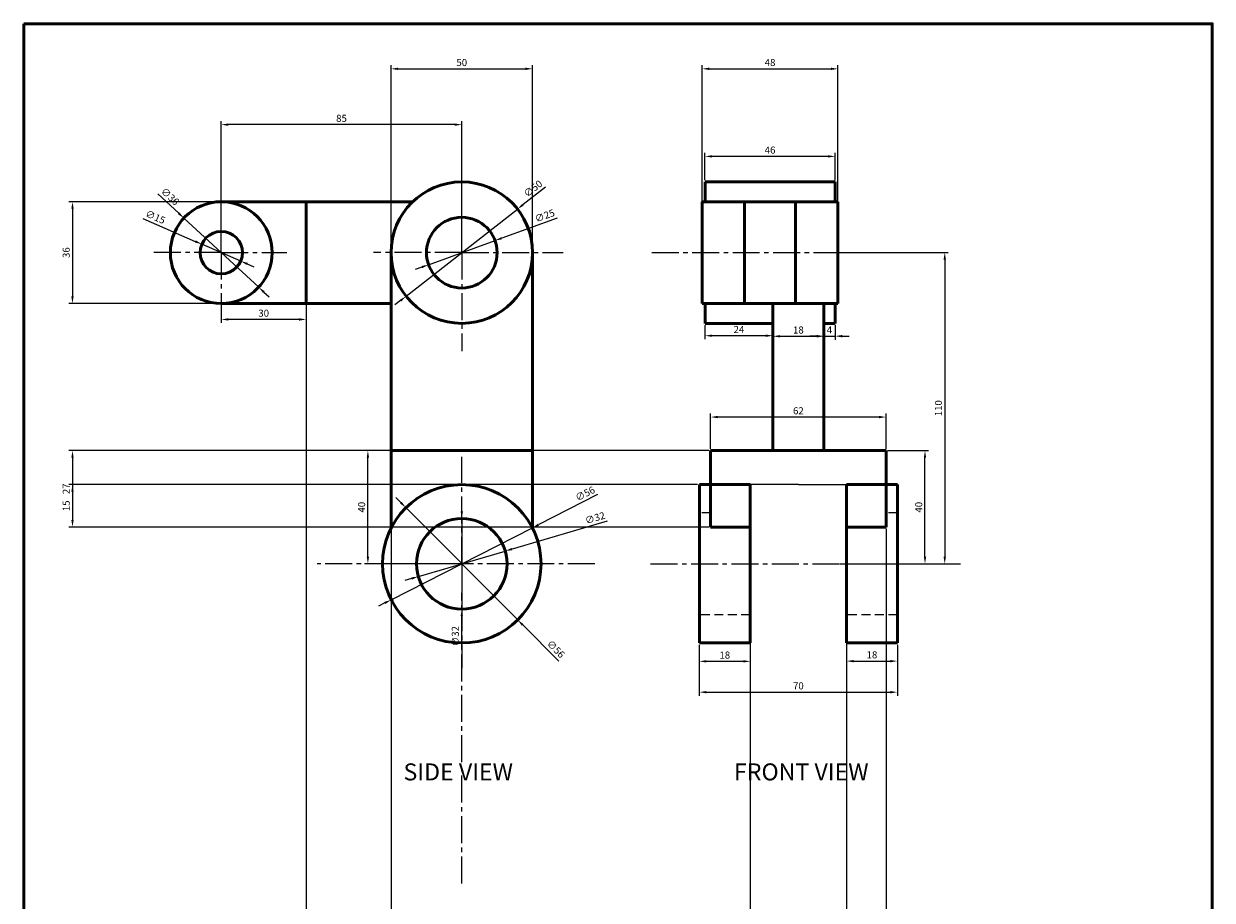
# Model space of a CAD drawing. Units: millimetres. Extents: x 1466 to 1886, y 5011 to 5605.
# Tile 4 of 4: x 1466 to 1886, y 5295 to 5605. Entities that reach past the tile are written whole.
import ezdxf

# ---------------------------------------------------------------- set-up
doc = ezdxf.new("R2010")
doc.units = ezdxf.units.MM
doc.linetypes.add('CENTER2', pattern=[28.575, 19.05, -3.175, 3.175, -3.175])
doc.linetypes.add('HIDDEN2', pattern=[4.7625, 3.175, -1.5875])
for name, color, linetype, lineweight in [('M-CNTR', 1, 'CENTER2', 18), ('M-DIMS', 2, 'Continuous', 25), ('M-HIDN', 4, 'HIDDEN2', 25), ('M-OUTL', 7, 'Continuous', 50), ('M-TEXT', 7, 'Continuous', 25), ('M-TTLB', 7, 'Continuous', 50)]:
    doc.layers.add(name, color=color, linetype=linetype, lineweight=lineweight)
doc.styles.get("Standard").update_dxf_attribs({"font": 'arial.ttf'})
doc.dimstyles.new('ISO-25', dxfattribs={"dimtxt": 2.5, "dimasz": 2.5, "dimexe": 1.25, "dimexo": 0.625, "dimtad": 1, "dimtxsty": 'Standard', "dimcen": 2.5, "dimadec": 0, "dimazin": 0, "dimtfac": 1, "dimtmove": 0, "dimatfit": 3, "dimfxl": 1, "dimarcsym": 0})

# ---------------------------------------------------------------- blocks, each defined once
blk = doc.blocks.new('*D26')
at = {"layer": 'Defpoints', "color": 0, "transparency": 16777216}
for p in [(1707.01, 5557.74), (1707.01, 5548.72), (1753.01, 5548.72)]:
    blk.add_point(p, dxfattribs=at)
at = {"layer": 'M-DIMS', "color": 0, "lineweight": -2, "transparency": 16777216}
for p, q in [((1707.01, 5549.34), (1707.01, 5558.99)), ((1750.51, 5557.74), (1709.51, 5557.74)), ((1753.01, 5549.34), (1753.01, 5558.99))]:
    blk.add_line(p, q, dxfattribs=at)
at = {"layer": 'M-DIMS', "color": 0, "transparency": 16777216}
for points in [[(1709.51, 5558.16), (1709.51, 5557.33), (1707.01, 5557.74)], [(1750.51, 5558.16), (1750.51, 5557.33), (1753.01, 5557.74)]]:
    blk.add_solid(points, dxfattribs=at)
at = {"layer": 'M-DIMS', "color": 0, "transparency": 16777216, "insert": (1730.01, 5559.65), "char_height": 2.5, "attachment_point": 5}
blk.add_mtext('46', dxfattribs=at)
blk = doc.blocks.new('*D27')
at = {"layer": 'Defpoints', "color": 0, "transparency": 16777216}
for p in [(1754.01, 5523.72), (1754.01, 5413.72), (1791.74, 5413.72)]:
    blk.add_point(p, dxfattribs=at)
at = {"layer": 'M-DIMS', "color": 0, "lineweight": -2, "transparency": 16777216}
for p, q in [((1754.64, 5523.72), (1792.99, 5523.72)), ((1791.74, 5521.22), (1791.74, 5416.22)), ((1754.64, 5413.72), (1792.99, 5413.72))]:
    blk.add_line(p, q, dxfattribs=at)
at = {"layer": 'M-DIMS', "color": 0, "transparency": 16777216}
for points in [[(1791.32, 5521.22), (1792.16, 5521.22), (1791.74, 5523.72)], [(1791.32, 5416.22), (1792.16, 5416.22), (1791.74, 5413.72)]]:
    blk.add_solid(points, dxfattribs=at)
at = {"layer": 'M-DIMS', "color": 0, "transparency": 16777216, "insert": (1789.84, 5468.72), "char_height": 2.5, "attachment_point": 5, "rotation": 90}
blk.add_mtext('110', dxfattribs=at)
blk = doc.blocks.new('*D28')
at = {"layer": 'Defpoints', "color": 0, "transparency": 16777216}
for p in [(1709.01, 5465.59), (1709.01, 5453.72), (1771.01, 5453.72)]:
    blk.add_point(p, dxfattribs=at)
at = {"layer": 'M-DIMS', "color": 0, "lineweight": -2, "transparency": 16777216}
for p, q in [((1709.01, 5454.34), (1709.01, 5466.84)), ((1768.51, 5465.59), (1711.51, 5465.59)), ((1771.01, 5454.34), (1771.01, 5466.84))]:
    blk.add_line(p, q, dxfattribs=at)
at = {"layer": 'M-DIMS', "color": 0, "transparency": 16777216}
for points in [[(1711.51, 5466), (1711.51, 5465.17), (1709.01, 5465.59)], [(1768.51, 5466), (1768.51, 5465.17), (1771.01, 5465.59)]]:
    blk.add_solid(points, dxfattribs=at)
at = {"layer": 'M-DIMS', "color": 0, "transparency": 16777216, "insert": (1740.01, 5467.49), "char_height": 2.5, "attachment_point": 5}
blk.add_mtext('62', dxfattribs=at)
blk = doc.blocks.new('*D29')
at = {"layer": 'Defpoints', "color": 0, "transparency": 16777216}
for p in [(1705.01, 5385.72), (1723.01, 5385.72), (1705.01, 5379.23)]:
    blk.add_point(p, dxfattribs=at)
at = {"layer": 'M-DIMS', "color": 0, "lineweight": -2, "transparency": 16777216}
for p, q in [((1705.01, 5385.09), (1705.01, 5377.98)), ((1723.01, 5385.09), (1723.01, 5377.98)), ((1720.51, 5379.23), (1707.51, 5379.23))]:
    blk.add_line(p, q, dxfattribs=at)
at = {"layer": 'M-DIMS', "color": 0, "transparency": 16777216}
for points in [[(1707.51, 5379.65), (1707.51, 5378.81), (1705.01, 5379.23)], [(1720.51, 5379.65), (1720.51, 5378.81), (1723.01, 5379.23)]]:
    blk.add_solid(points, dxfattribs=at)
at = {"layer": 'M-DIMS', "color": 0, "transparency": 16777216, "insert": (1714.01, 5381.13), "char_height": 2.5, "attachment_point": 5}
blk.add_mtext('18', dxfattribs=at)
blk = doc.blocks.new('*D30')
at = {"layer": 'Defpoints', "color": 0, "transparency": 16777216}
for p in [(1757.01, 5385.72), (1775.01, 5385.72), (1775.01, 5379.31)]:
    blk.add_point(p, dxfattribs=at)
at = {"layer": 'M-DIMS', "color": 0, "lineweight": -2, "transparency": 16777216}
for p, q in [((1757.01, 5385.09), (1757.01, 5378.06)), ((1775.01, 5385.09), (1775.01, 5378.06)), ((1759.51, 5379.31), (1772.51, 5379.31))]:
    blk.add_line(p, q, dxfattribs=at)
at = {"layer": 'M-DIMS', "color": 0, "transparency": 16777216}
for points in [[(1759.51, 5379.72), (1759.51, 5378.89), (1757.01, 5379.31)], [(1772.51, 5379.72), (1772.51, 5378.89), (1775.01, 5379.31)]]:
    blk.add_solid(points, dxfattribs=at)
at = {"layer": 'M-DIMS', "color": 0, "transparency": 16777216, "insert": (1766.01, 5381.21), "char_height": 2.5, "attachment_point": 5}
blk.add_mtext('18', dxfattribs=at)
blk = doc.blocks.new('*D31')
at = {"layer": 'Defpoints', "color": 0, "transparency": 16777216}
for p in [(1705.01, 5385.72), (1775.01, 5385.72), (1775.01, 5368.33)]:
    blk.add_point(p, dxfattribs=at)
at = {"layer": 'M-DIMS', "color": 0, "lineweight": -2, "transparency": 16777216}
for p, q in [((1705.01, 5385.09), (1705.01, 5367.08)), ((1775.01, 5385.09), (1775.01, 5367.08)), ((1707.51, 5368.33), (1772.51, 5368.33))]:
    blk.add_line(p, q, dxfattribs=at)
at = {"layer": 'M-DIMS', "color": 0, "transparency": 16777216}
for points in [[(1707.51, 5368.74), (1707.51, 5367.91), (1705.01, 5368.33)], [(1772.51, 5368.74), (1772.51, 5367.91), (1775.01, 5368.33)]]:
    blk.add_solid(points, dxfattribs=at)
at = {"layer": 'M-DIMS', "color": 0, "transparency": 16777216, "insert": (1740.01, 5370.23), "char_height": 2.5, "attachment_point": 5}
blk.add_mtext('70', dxfattribs=at)
blk = doc.blocks.new('*D32')
at = {"layer": 'Defpoints', "color": 0, "transparency": 16777216}
for p in [(1771.01, 5453.72), (1784.76, 5453.72), (1775.01, 5413.72)]:
    blk.add_point(p, dxfattribs=at)
at = {"layer": 'M-DIMS', "color": 0, "lineweight": -2, "transparency": 16777216}
for p, q in [((1771.64, 5453.72), (1786.01, 5453.72)), ((1784.76, 5416.22), (1784.76, 5451.22)), ((1775.64, 5413.72), (1786.01, 5413.72))]:
    blk.add_line(p, q, dxfattribs=at)
at = {"layer": 'M-DIMS', "color": 0, "transparency": 16777216}
for points in [[(1784.35, 5451.22), (1785.18, 5451.22), (1784.76, 5453.72)], [(1784.35, 5416.22), (1785.18, 5416.22), (1784.76, 5413.72)]]:
    blk.add_solid(points, dxfattribs=at)
at = {"layer": 'M-DIMS', "color": 0, "transparency": 16777216, "insert": (1782.86, 5433.72), "char_height": 2.5, "attachment_point": 5, "rotation": 90}
blk.add_mtext('40', dxfattribs=at)
blk = doc.blocks.new('*D33')
at = {"layer": 'Defpoints', "color": 0, "transparency": 16777216}
for p in [(1707.01, 5498.72), (1731.01, 5498.72), (1707.01, 5494.35)]:
    blk.add_point(p, dxfattribs=at)
at = {"layer": 'M-DIMS', "color": 0, "lineweight": -2, "transparency": 16777216}
for p, q in [((1707.01, 5498.09), (1707.01, 5493.1)), ((1731.01, 5498.09), (1731.01, 5493.1)), ((1728.51, 5494.35), (1709.51, 5494.35))]:
    blk.add_line(p, q, dxfattribs=at)
at = {"layer": 'M-DIMS', "color": 0, "transparency": 16777216}
for points in [[(1709.51, 5494.77), (1709.51, 5493.94), (1707.01, 5494.35)], [(1728.51, 5494.77), (1728.51, 5493.94), (1731.01, 5494.35)]]:
    blk.add_solid(points, dxfattribs=at)
at = {"layer": 'M-DIMS', "color": 0, "transparency": 16777216, "insert": (1719.01, 5496.23), "char_height": 2.5, "attachment_point": 5}
blk.add_mtext('24', dxfattribs=at)
blk = doc.blocks.new('*D34')
at = {"layer": 'Defpoints', "color": 0, "transparency": 16777216}
for p in [(1731.01, 5498.72), (1749.01, 5498.72), (1749.01, 5494.15)]:
    blk.add_point(p, dxfattribs=at)
at = {"layer": 'M-DIMS', "color": 0, "lineweight": -2, "transparency": 16777216}
for p, q in [((1731.01, 5498.09), (1731.01, 5492.9)), ((1749.01, 5498.09), (1749.01, 5492.9)), ((1733.51, 5494.15), (1746.51, 5494.15))]:
    blk.add_line(p, q, dxfattribs=at)
at = {"layer": 'M-DIMS', "color": 0, "transparency": 16777216}
for points in [[(1733.51, 5494.56), (1733.51, 5493.73), (1731.01, 5494.15)], [(1746.51, 5494.56), (1746.51, 5493.73), (1749.01, 5494.15)]]:
    blk.add_solid(points, dxfattribs=at)
at = {"layer": 'M-DIMS', "color": 0, "transparency": 16777216, "insert": (1740.01, 5496.05), "char_height": 2.5, "attachment_point": 5}
blk.add_mtext('18', dxfattribs=at)
blk = doc.blocks.new('*D35')
at = {"layer": 'Defpoints', "color": 0, "transparency": 16777216}
for p in [(1749.01, 5498.72), (1753.01, 5498.72), (1753.01, 5494.19)]:
    blk.add_point(p, dxfattribs=at)
at = {"layer": 'M-DIMS', "color": 0, "lineweight": -2, "transparency": 16777216}
for p, q in [((1749.01, 5498.09), (1749.01, 5492.94)), ((1753.01, 5498.09), (1753.01, 5492.94)), ((1746.51, 5494.19), (1744.01, 5494.19)), ((1749.01, 5494.19), (1753.01, 5494.19)), ((1755.51, 5494.19), (1758.01, 5494.19))]:
    blk.add_line(p, q, dxfattribs=at)
at = {"layer": 'M-DIMS', "color": 0, "transparency": 16777216}
for points in [[(1746.51, 5494.61), (1746.51, 5493.77), (1749.01, 5494.19)], [(1755.51, 5494.61), (1755.51, 5493.77), (1753.01, 5494.19)]]:
    blk.add_solid(points, dxfattribs=at)
at = {"layer": 'M-DIMS', "color": 0, "transparency": 16777216, "insert": (1751.01, 5496.06), "char_height": 2.5, "attachment_point": 5}
blk.add_mtext('4', dxfattribs=at)
blk = doc.blocks.new('*D36')
at = {"layer": 'Defpoints', "color": 0, "transparency": 16777216}
for p in [(1522.85, 5535.94), (1549.28, 5511.49)]:
    blk.add_point(p, dxfattribs=at)
at = {"layer": 'M-DIMS', "color": 0, "lineweight": -2, "transparency": 16777216}
for p, q in [((1513.64, 5544.46), (1521.02, 5537.64)), ((1549.28, 5511.49), (1522.85, 5535.94)), ((1551.11, 5509.79), (1552.95, 5508.1))]:
    blk.add_line(p, q, dxfattribs=at)
at = {"layer": 'M-DIMS', "color": 0, "transparency": 16777216}
for points in [[(1521.3, 5537.94), (1520.73, 5537.33), (1522.85, 5535.94)], [(1551.4, 5510.1), (1550.83, 5509.49), (1549.28, 5511.49)]]:
    blk.add_solid(points, dxfattribs=at)
at = {"layer": 'M-DIMS', "color": 0, "transparency": 16777216, "insert": (1517.75, 5543.35), "char_height": 2.5, "attachment_point": 5, "rotation": 317.2254}
blk.add_mtext('∅36', dxfattribs=at)
blk = doc.blocks.new('*D37')
at = {"layer": 'Defpoints', "color": 0, "transparency": 16777216}
for p in [(1529.19, 5526.7), (1542.94, 5520.73)]:
    blk.add_point(p, dxfattribs=at)
at = {"layer": 'M-DIMS', "color": 0, "lineweight": -2, "transparency": 16777216}
for p, q in [((1508.4, 5535.73), (1526.89, 5527.7)), ((1542.94, 5520.73), (1529.19, 5526.7)), ((1545.24, 5519.73), (1547.53, 5518.74))]:
    blk.add_line(p, q, dxfattribs=at)
at = {"layer": 'M-DIMS', "color": 0, "transparency": 16777216}
for points in [[(1527.06, 5528.08), (1526.73, 5527.32), (1529.19, 5526.7)], [(1545.4, 5520.12), (1545.07, 5519.35), (1542.94, 5520.73)]]:
    blk.add_solid(points, dxfattribs=at)
at = {"layer": 'M-DIMS', "color": 0, "transparency": 16777216, "insert": (1512.66, 5536.03), "char_height": 2.5, "attachment_point": 5, "rotation": 336.5262}
blk.add_mtext('∅15', dxfattribs=at)
blk = doc.blocks.new('*D38')
at = {"layer": 'Defpoints', "color": 0, "transparency": 16777216}
for p in [(1640.74, 5539.13), (1601.39, 5508.3)]:
    blk.add_point(p, dxfattribs=at)
at = {"layer": 'M-DIMS', "color": 0, "lineweight": -2, "transparency": 16777216}
for p, q in [((1650.62, 5546.87), (1642.71, 5540.68)), ((1601.39, 5508.3), (1640.74, 5539.13)), ((1599.42, 5506.76), (1597.45, 5505.21))]:
    blk.add_line(p, q, dxfattribs=at)
at = {"layer": 'M-DIMS', "color": 0, "transparency": 16777216}
for points in [[(1642.46, 5541), (1642.97, 5540.35), (1640.74, 5539.13)], [(1599.16, 5507.08), (1599.67, 5506.43), (1601.39, 5508.3)]]:
    blk.add_solid(points, dxfattribs=at)
at = {"layer": 'M-DIMS', "color": 0, "transparency": 16777216, "insert": (1646.43, 5546.1), "char_height": 2.5, "attachment_point": 5, "rotation": 38.0777}
blk.add_mtext('∅50', dxfattribs=at)
blk = doc.blocks.new('*D39')
at = {"layer": 'Defpoints', "color": 0, "transparency": 16777216}
for p in [(1632.82, 5527.98), (1609.31, 5519.46)]:
    blk.add_point(p, dxfattribs=at)
at = {"layer": 'M-DIMS', "color": 0, "lineweight": -2, "transparency": 16777216}
for p, q in [((1654.71, 5535.91), (1635.17, 5528.83)), ((1609.31, 5519.46), (1632.82, 5527.98)), ((1606.96, 5518.61), (1604.61, 5517.75))]:
    blk.add_line(p, q, dxfattribs=at)
at = {"layer": 'M-DIMS', "color": 0, "transparency": 16777216}
for points in [[(1635.03, 5529.22), (1635.31, 5528.44), (1632.82, 5527.98)], [(1606.82, 5519), (1607.1, 5518.21), (1609.31, 5519.46)]]:
    blk.add_solid(points, dxfattribs=at)
at = {"layer": 'M-DIMS', "color": 0, "transparency": 16777216, "insert": (1650.48, 5536.47), "char_height": 2.5, "attachment_point": 5, "rotation": 19.9205}
blk.add_mtext('∅25', dxfattribs=at)
blk = doc.blocks.new('*D40')
at = {"layer": 'Defpoints', "color": 0, "transparency": 16777216}
for p in [(1646.01, 5426.43), (1596.12, 5401)]:
    blk.add_point(p, dxfattribs=at)
at = {"layer": 'M-DIMS', "color": 0, "lineweight": -2, "transparency": 16777216}
for p, q in [((1669.04, 5438.18), (1648.24, 5427.57)), ((1596.12, 5401), (1646.01, 5426.43)), ((1593.89, 5399.86), (1591.67, 5398.73))]:
    blk.add_line(p, q, dxfattribs=at)
at = {"layer": 'M-DIMS', "color": 0, "transparency": 16777216}
for points in [[(1648.05, 5427.94), (1648.43, 5427.2), (1646.01, 5426.43)], [(1593.7, 5400.23), (1594.08, 5399.49), (1596.12, 5401)]]:
    blk.add_solid(points, dxfattribs=at)
at = {"layer": 'M-DIMS', "color": 0, "transparency": 16777216, "insert": (1664.78, 5438.22), "char_height": 2.5, "attachment_point": 5, "rotation": 27.0155}
blk.add_mtext('∅56', dxfattribs=at)
blk = doc.blocks.new('*D41')
at = {"layer": 'Defpoints', "color": 0, "transparency": 16777216}
for p in [(1636.42, 5418.22), (1605.71, 5409.21)]:
    blk.add_point(p, dxfattribs=at)
at = {"layer": 'M-DIMS', "color": 0, "lineweight": -2, "transparency": 16777216}
for p, q in [((1672.42, 5428.79), (1638.82, 5418.93)), ((1605.71, 5409.21), (1636.42, 5418.22)), ((1603.31, 5408.51), (1600.91, 5407.8))]:
    blk.add_line(p, q, dxfattribs=at)
at = {"layer": 'M-DIMS', "color": 0, "transparency": 16777216}
for points in [[(1638.7, 5419.33), (1638.93, 5418.53), (1636.42, 5418.22)], [(1603.2, 5408.91), (1603.43, 5408.11), (1605.71, 5409.21)]]:
    blk.add_solid(points, dxfattribs=at)
at = {"layer": 'M-DIMS', "color": 0, "transparency": 16777216, "insert": (1668.25, 5429.62), "char_height": 2.5, "attachment_point": 5, "rotation": 16.3589}
blk.add_mtext('∅32', dxfattribs=at)
blk = doc.blocks.new('*D42')
at = {"layer": 'Defpoints', "color": 0, "transparency": 16777216}
for p in [(1536.06, 5505.72), (1566.06, 5505.72), (1536.06, 5500.1)]:
    blk.add_point(p, dxfattribs=at)
at = {"layer": 'M-DIMS', "color": 0, "lineweight": -2, "transparency": 16777216}
for p, q in [((1536.06, 5505.09), (1536.06, 5498.85)), ((1566.06, 5505.09), (1566.06, 5498.85)), ((1563.56, 5500.1), (1538.56, 5500.1))]:
    blk.add_line(p, q, dxfattribs=at)
at = {"layer": 'M-DIMS', "color": 0, "transparency": 16777216}
for points in [[(1538.56, 5500.52), (1538.56, 5499.68), (1536.06, 5500.1)], [(1563.56, 5500.52), (1563.56, 5499.68), (1566.06, 5500.1)]]:
    blk.add_solid(points, dxfattribs=at)
at = {"layer": 'M-DIMS', "color": 0, "transparency": 16777216, "insert": (1551.06, 5502), "char_height": 2.5, "attachment_point": 5}
blk.add_mtext('30', dxfattribs=at)
blk = doc.blocks.new('*D43')
at = {"layer": 'Defpoints', "color": 0, "transparency": 16777216}
for p in [(1536.06, 5568.97), (1536.06, 5523.72), (1621.06, 5523.72)]:
    blk.add_point(p, dxfattribs=at)
at = {"layer": 'M-DIMS', "color": 0, "lineweight": -2, "transparency": 16777216}
for p, q in [((1536.06, 5524.34), (1536.06, 5570.22)), ((1621.06, 5524.34), (1621.06, 5570.22)), ((1618.56, 5568.97), (1538.56, 5568.97))]:
    blk.add_line(p, q, dxfattribs=at)
at = {"layer": 'M-DIMS', "color": 0, "transparency": 16777216}
for points in [[(1538.56, 5569.38), (1538.56, 5568.55), (1536.06, 5568.97)], [(1618.56, 5569.38), (1618.56, 5568.55), (1621.06, 5568.97)]]:
    blk.add_solid(points, dxfattribs=at)
at = {"layer": 'M-DIMS', "color": 0, "transparency": 16777216, "insert": (1578.56, 5570.87), "char_height": 2.5, "attachment_point": 5}
blk.add_mtext('85', dxfattribs=at)
blk = doc.blocks.new('*D44')
at = {"layer": 'Defpoints', "color": 0, "transparency": 16777216}
for p in [(1587.88, 5453.72), (1621.06, 5453.72), (1621.06, 5413.72)]:
    blk.add_point(p, dxfattribs=at)
at = {"layer": 'M-DIMS', "color": 0, "lineweight": -2, "transparency": 16777216}
for p, q in [((1620.44, 5453.72), (1586.63, 5453.72)), ((1587.88, 5416.22), (1587.88, 5451.22)), ((1620.44, 5413.72), (1586.63, 5413.72))]:
    blk.add_line(p, q, dxfattribs=at)
at = {"layer": 'M-DIMS', "color": 0, "transparency": 16777216}
for points in [[(1587.46, 5451.22), (1588.29, 5451.22), (1587.88, 5453.72)], [(1587.46, 5416.22), (1588.29, 5416.22), (1587.88, 5413.72)]]:
    blk.add_solid(points, dxfattribs=at)
at = {"layer": 'M-DIMS', "color": 0, "transparency": 16777216, "insert": (1585.98, 5433.72), "char_height": 2.5, "attachment_point": 5, "rotation": 90}
blk.add_mtext('40', dxfattribs=at)
blk = doc.blocks.new('*D53')
at = {"layer": 'Defpoints', "color": 0, "transparency": 16777216}
for p in [(1566.06, 5541.72), (1483.48, 5505.72), (1566.06, 5505.72)]:
    blk.add_point(p, dxfattribs=at)
at = {"layer": 'M-DIMS', "color": 0, "lineweight": -2, "transparency": 16777216}
for p, q in [((1565.44, 5541.72), (1482.23, 5541.72)), ((1483.48, 5539.22), (1483.48, 5508.22)), ((1565.44, 5505.72), (1482.23, 5505.72))]:
    blk.add_line(p, q, dxfattribs=at)
at = {"layer": 'M-DIMS', "color": 0, "transparency": 16777216}
for points in [[(1483.07, 5539.22), (1483.9, 5539.22), (1483.48, 5541.72)], [(1483.07, 5508.22), (1483.9, 5508.22), (1483.48, 5505.72)]]:
    blk.add_solid(points, dxfattribs=at)
at = {"layer": 'M-DIMS', "color": 0, "transparency": 16777216, "insert": (1481.58, 5523.72), "char_height": 2.5, "attachment_point": 5, "rotation": 90}
blk.add_mtext('36', dxfattribs=at)
blk = doc.blocks.new('*D54')
at = {"layer": 'Defpoints', "color": 0, "transparency": 16777216}
for p in [(1566.06, 5505.72), (1596.06, 5505.72), (1596.06, 5011.83)]:
    blk.add_point(p, dxfattribs=at)
at = {"layer": 'M-DIMS', "color": 0, "lineweight": -2, "transparency": 16777216}
for p, q in [((1566.06, 5505.09), (1566.06, 5010.58)), ((1596.06, 5505.09), (1596.06, 5010.58)), ((1568.56, 5011.83), (1593.56, 5011.83))]:
    blk.add_line(p, q, dxfattribs=at)
at = {"layer": 'M-DIMS', "color": 0, "transparency": 16777216}
for points in [[(1568.56, 5012.25), (1568.56, 5011.41), (1566.06, 5011.83)], [(1593.56, 5012.25), (1593.56, 5011.41), (1596.06, 5011.83)]]:
    blk.add_solid(points, dxfattribs=at)
at = {"layer": 'M-DIMS', "color": 0, "transparency": 16777216, "insert": (1581.06, 5013.73), "char_height": 2.5, "attachment_point": 5}
blk.add_mtext('30', dxfattribs=at)
blk = doc.blocks.new('*D55')
at = {"layer": 'Defpoints', "color": 0, "transparency": 16777216}
for p in [(1646.06, 5588.7), (1596.06, 5453.72), (1646.06, 5453.72)]:
    blk.add_point(p, dxfattribs=at)
at = {"layer": 'M-DIMS', "color": 0, "lineweight": -2, "transparency": 16777216}
for p, q in [((1596.06, 5454.34), (1596.06, 5589.95)), ((1598.56, 5588.7), (1643.56, 5588.7)), ((1646.06, 5454.34), (1646.06, 5589.95))]:
    blk.add_line(p, q, dxfattribs=at)
at = {"layer": 'M-DIMS', "color": 0, "transparency": 16777216}
for points in [[(1598.56, 5589.12), (1598.56, 5588.29), (1596.06, 5588.7)], [(1643.56, 5589.12), (1643.56, 5588.29), (1646.06, 5588.7)]]:
    blk.add_solid(points, dxfattribs=at)
at = {"layer": 'M-DIMS', "color": 0, "transparency": 16777216, "insert": (1621.06, 5590.6), "char_height": 2.5, "attachment_point": 5}
blk.add_mtext('50', dxfattribs=at)
blk = doc.blocks.new('*D56')
at = {"layer": 'Defpoints', "color": 0, "transparency": 16777216}
for p in [(1754.01, 5588.7), (1706.01, 5505.72), (1754.01, 5505.72)]:
    blk.add_point(p, dxfattribs=at)
at = {"layer": 'M-DIMS', "color": 0, "lineweight": -2, "transparency": 16777216}
for p, q in [((1706.01, 5506.34), (1706.01, 5589.95)), ((1708.51, 5588.7), (1751.51, 5588.7)), ((1754.01, 5506.34), (1754.01, 5589.95))]:
    blk.add_line(p, q, dxfattribs=at)
at = {"layer": 'M-DIMS', "color": 0, "transparency": 16777216}
for points in [[(1708.51, 5589.12), (1708.51, 5588.29), (1706.01, 5588.7)], [(1751.51, 5589.12), (1751.51, 5588.29), (1754.01, 5588.7)]]:
    blk.add_solid(points, dxfattribs=at)
at = {"layer": 'M-DIMS', "color": 0, "transparency": 16777216, "insert": (1730.01, 5590.6), "char_height": 2.5, "attachment_point": 5}
blk.add_mtext('48', dxfattribs=at)
blk = doc.blocks.new('*D57')
at = {"layer": 'Defpoints', "color": 0, "transparency": 16777216}
for p in [(1723.01, 5426.72), (1757.01, 5426.72), (1757.01, 5011.83)]:
    blk.add_point(p, dxfattribs=at)
at = {"layer": 'M-DIMS', "color": 0, "lineweight": -2, "transparency": 16777216}
for p, q in [((1723.01, 5426.09), (1723.01, 5010.58)), ((1757.01, 5426.09), (1757.01, 5010.58)), ((1725.51, 5011.83), (1754.51, 5011.83))]:
    blk.add_line(p, q, dxfattribs=at)
at = {"layer": 'M-DIMS', "color": 0, "transparency": 16777216}
for points in [[(1725.51, 5012.25), (1725.51, 5011.41), (1723.01, 5011.83)], [(1754.51, 5012.25), (1754.51, 5011.41), (1757.01, 5011.83)]]:
    blk.add_solid(points, dxfattribs=at)
at = {"layer": 'M-DIMS', "color": 0, "transparency": 16777216, "insert": (1740.01, 5013.73), "char_height": 2.5, "attachment_point": 5}
blk.add_mtext('34', dxfattribs=at)
blk = doc.blocks.new('*D58')
at = {"layer": 'Defpoints', "color": 0, "transparency": 16777216}
for p in [(1757.01, 5426.72), (1771.01, 5426.72), (1771.01, 5011.83)]:
    blk.add_point(p, dxfattribs=at)
at = {"layer": 'M-DIMS', "color": 0, "lineweight": -2, "transparency": 16777216}
for p, q in [((1757.01, 5426.09), (1757.01, 5010.58)), ((1771.01, 5426.09), (1771.01, 5010.58)), ((1759.51, 5011.83), (1768.51, 5011.83))]:
    blk.add_line(p, q, dxfattribs=at)
at = {"layer": 'M-DIMS', "color": 0, "transparency": 16777216}
for points in [[(1759.51, 5012.25), (1759.51, 5011.41), (1757.01, 5011.83)], [(1768.51, 5012.25), (1768.51, 5011.41), (1771.01, 5011.83)]]:
    blk.add_solid(points, dxfattribs=at)
at = {"layer": 'M-DIMS', "color": 0, "transparency": 16777216, "insert": (1764.01, 5013.71), "char_height": 2.5, "attachment_point": 5}
blk.add_mtext('14', dxfattribs=at)
blk = doc.blocks.new('*D59')
at = {"layer": 'Defpoints', "color": 0, "transparency": 16777216}
for p in [(1709.01, 5453.72), (1483.48, 5426.72), (1709.01, 5426.72)]:
    blk.add_point(p, dxfattribs=at)
at = {"layer": 'M-DIMS', "color": 0, "lineweight": -2, "transparency": 16777216}
for p, q in [((1708.39, 5453.72), (1482.23, 5453.72)), ((1483.48, 5451.22), (1483.48, 5429.22)), ((1708.39, 5426.72), (1482.23, 5426.72))]:
    blk.add_line(p, q, dxfattribs=at)
at = {"layer": 'M-DIMS', "color": 0, "transparency": 16777216}
for points in [[(1483.07, 5451.22), (1483.9, 5451.22), (1483.48, 5453.72)], [(1483.07, 5429.22), (1483.9, 5429.22), (1483.48, 5426.72)]]:
    blk.add_solid(points, dxfattribs=at)
at = {"layer": 'M-DIMS', "color": 0, "transparency": 16777216, "insert": (1481.6, 5440.22), "char_height": 2.5, "attachment_point": 5, "rotation": 90}
blk.add_mtext('27', dxfattribs=at)
blk = doc.blocks.new('*D60')
at = {"layer": 'Defpoints', "color": 0, "transparency": 16777216}
for p in [(1705.01, 5441.72), (1483.48, 5426.72), (1709.01, 5426.72)]:
    blk.add_point(p, dxfattribs=at)
at = {"layer": 'M-DIMS', "color": 0, "lineweight": -2, "transparency": 16777216}
for p, q in [((1704.39, 5441.72), (1482.23, 5441.72)), ((1483.48, 5439.22), (1483.48, 5429.22)), ((1708.39, 5426.72), (1482.23, 5426.72))]:
    blk.add_line(p, q, dxfattribs=at)
at = {"layer": 'M-DIMS', "color": 0, "transparency": 16777216}
for points in [[(1483.07, 5439.22), (1483.9, 5439.22), (1483.48, 5441.72)], [(1483.07, 5429.22), (1483.9, 5429.22), (1483.48, 5426.72)]]:
    blk.add_solid(points, dxfattribs=at)
at = {"layer": 'M-DIMS', "color": 0, "transparency": 16777216, "insert": (1481.58, 5434.22), "char_height": 2.5, "attachment_point": 5, "rotation": 90}
blk.add_mtext('15', dxfattribs=at)
blk = doc.blocks.new('*D61')
at = {"layer": 'Defpoints', "color": 0, "transparency": 16777216}
for p in [(1601.31, 5433.56), (1640.82, 5393.88)]:
    blk.add_point(p, dxfattribs=at)
at = {"layer": 'M-DIMS', "color": 0, "lineweight": -2, "transparency": 16777216}
for p, q in [((1599.54, 5435.33), (1597.78, 5437.1)), ((1601.31, 5433.56), (1640.82, 5393.88)), ((1655.34, 5379.3), (1642.59, 5392.11))]:
    blk.add_line(p, q, dxfattribs=at)
at = {"layer": 'M-DIMS', "color": 0, "transparency": 16777216}
for points in [[(1599.84, 5435.62), (1599.25, 5435.03), (1601.31, 5433.56)], [(1642.88, 5392.4), (1642.29, 5391.81), (1640.82, 5393.88)]]:
    blk.add_solid(points, dxfattribs=at)
at = {"layer": 'M-DIMS', "color": 0, "transparency": 16777216, "insert": (1654.07, 5383.36), "char_height": 2.5, "attachment_point": 5, "rotation": 314.8826}
blk.add_mtext('∅56', dxfattribs=at)
blk = doc.blocks.new('*D62')
at = {"layer": 'Defpoints', "color": 0, "transparency": 16777216}
for p in [(1621.07, 5429.72), (1621.06, 5397.72)]:
    blk.add_point(p, dxfattribs=at)
at = {"layer": 'M-DIMS', "color": 0, "lineweight": -2, "transparency": 16777216}
for p, q in [((1621.07, 5432.22), (1621.07, 5434.72)), ((1621.07, 5429.72), (1621.06, 5397.72)), ((1621.06, 5384.35), (1621.06, 5395.22))]:
    blk.add_line(p, q, dxfattribs=at)
at = {"layer": 'M-DIMS', "color": 0, "transparency": 16777216}
for points in [[(1620.65, 5432.22), (1621.49, 5432.22), (1621.07, 5429.72)], [(1620.64, 5395.22), (1621.48, 5395.22), (1621.06, 5397.72)]]:
    blk.add_solid(points, dxfattribs=at)
at = {"layer": 'M-DIMS', "color": 0, "transparency": 16777216, "insert": (1619.09, 5388.12), "char_height": 2.5, "attachment_point": 5, "rotation": 89.9831}
blk.add_mtext('∅32', dxfattribs=at)

msp = doc.modelspace()

# ---------------------------------------------------------------- linework, layer by layer
at = {"layer": 'M-CNTR', "ltscale": 0.5}
for p, q in [((1621.065, 5523.716), (1621.065, 5560.702)), ((1536.065, 5523.716), (1536.065, 5550.917)), ((1536.065, 5523.716), (1511.482, 5523.716)), ((1536.065, 5523.716), (1559.27, 5523.716)), ((1536.065, 5523.716), (1536.065, 5500.1)), ((1621.065, 5523.716), (1589.806, 5523.716)), ((1621.065, 5523.716), (1656.937, 5523.716)), ((1621.065, 5523.716), (1621.065, 5488.872)), ((1688.23, 5523.716), (1770.393, 5523.716)), ((1621.065, 5413.716), (1621.065, 5451.562)), ((1668.049, 5413.716), (1570.004, 5413.716)), ((1621.065, 5413.716), (1621.065, 5376.768)), ((1687.799, 5413.716), (1797.336, 5413.716)), ((1621.065, 5300.716), (1621.065, 5403.5))]:
    msp.add_line(p, q, dxfattribs=at)
at = {"layer": 'M-CNTR'}
for q in [(1723.014, 5441.716), (1757.014, 5441.716)]:
    msp.add_line((1740.014, 5441.716), q, dxfattribs=at)
at = {"layer": 'M-HIDN'}
for p, q in [((1709.014, 5431.716), (1705.014, 5431.716)), ((1775.014, 5431.716), (1771.014, 5431.716)), ((1723.014, 5395.716), (1705.014, 5395.716)), ((1775.014, 5395.716), (1757.014, 5395.716))]:
    msp.add_line(p, q, dxfattribs=at)
at = {"layer": 'M-OUTL'}
for p, q in [((1753.014, 5548.716), (1707.014, 5548.716)), ((1707.014, 5548.716), (1707.014, 5541.716)), ((1753.014, 5548.716), (1753.014, 5541.716)), ((1603.715, 5541.716), (1536.065, 5541.716)), ((1566.065, 5541.716), (1566.065, 5505.716)), ((1706.014, 5541.716), (1754.014, 5541.716)), ((1706.014, 5541.716), (1706.014, 5505.716)), ((1721.014, 5541.716), (1721.014, 5505.716)), ((1739.014, 5541.716), (1739.014, 5505.716)), ((1754.014, 5505.716), (1754.014, 5541.716)), ((1596.065, 5426.326), (1596.065, 5523.716)), ((1646.065, 5426.326), (1646.065, 5523.716)), ((1596.065, 5505.716), (1536.065, 5505.716)), ((1706.014, 5505.716), (1754.014, 5505.716)), ((1707.014, 5505.716), (1707.014, 5498.716)), ((1731.014, 5453.716), (1731.014, 5505.716)), ((1749.014, 5453.716), (1749.014, 5505.716)), ((1753.014, 5498.716), (1753.014, 5505.716)), ((1731.014, 5498.716), (1707.014, 5498.716)), ((1753.014, 5498.716), (1749.014, 5498.716)), ((1621.065, 5453.716), (1596.065, 5453.716)), ((1621.065, 5453.716), (1646.065, 5453.716)), ((1771.014, 5453.716), (1709.014, 5453.716)), ((1709.014, 5426.716), (1709.014, 5453.716)), ((1771.014, 5453.716), (1771.014, 5426.716)), ((1705.014, 5385.716), (1705.014, 5441.716)), ((1705.014, 5441.716), (1723.014, 5441.716)), ((1723.014, 5441.716), (1723.014, 5385.716)), ((1757.014, 5385.716), (1757.014, 5441.716)), ((1757.014, 5441.716), (1775.014, 5441.716)), ((1775.014, 5441.716), (1775.014, 5385.716)), ((1723.014, 5426.716), (1709.014, 5426.716)), ((1771.014, 5426.716), (1757.014, 5426.716)), ((1705.014, 5385.716), (1723.014, 5385.716)), ((1775.014, 5385.716), (1757.014, 5385.716))]:
    msp.add_line(p, q, dxfattribs=at)
for centre, radius in [((1621.065, 5523.716), 25), ((1536.065, 5523.716), 18), ((1621.065, 5523.716), 12.5), ((1536.065, 5523.716), 7.5), ((1621.065, 5413.716), 28), ((1621.065, 5413.716), 16)]:
    msp.add_circle(centre, radius, dxfattribs=at)
at = {"layer": 'M-TTLB'}
msp.add_lwpolyline([(1466.267, 5604.631), (1886.267, 5604.631), (1886.267, 5010.631), (1466.267, 5010.631)], close=True, dxfattribs=at)

# ---------------------------------------------------------------- texts
at = {"layer": 'M-TEXT', "char_height": 6, "attachment_point": 1}
for s, width, insert in [('SIDE VIEW', 63.12046, (1600.47, 5343.144)), ('FRONT VIEW', 52.67199, (1717.262, 5343.148))]:
    msp.add_mtext_dynamic_manual_height_columns(s, width=width, gutter_width=12.5, heights=[0], dxfattribs=dict(at, insert=insert))

# ---------------------------------------------------------------- dimensions: what is measured, and where the dimension line sits
at = {"layer": 'M-DIMS'}
for base, p1, p2, override, picture, middle in [((1646.065, 5588.702), (1596.065, 5453.716), (1646.065, 5453.716), {"dimdec": 0, "dimlfac": 1, "dimrnd": 0, "dimzin": 0, "dimdsep": 46, "dimlunit": 2}, '*D55', (1621.065, 5590.603)), ((1754.014, 5588.702), (1706.014, 5505.716), (1754.014, 5505.716), {"dimdec": 0, "dimlfac": 1, "dimrnd": 0, "dimzin": 0, "dimdsep": 46, "dimlunit": 2}, '*D56', (1730.014, 5590.603)), ((1536.065, 5568.968), (1621.065, 5523.716), (1536.065, 5523.716), {"dimclrd": 0, "dimclre": 0, "dimclrt": 0}, '*D43', (1578.565, 5570.869)), ((1707.014, 5557.744), (1753.014, 5548.716), (1707.014, 5548.716), {"dimclrd": 0, "dimclre": 0, "dimclrt": 0}, '*D26', (1730.014, 5559.646)), ((1536.065, 5500.1), (1566.065, 5505.716), (1536.065, 5505.716), {"dimclrd": 0, "dimclre": 0, "dimclrt": 0}, '*D42', (1551.065, 5502.003)), ((1596.065, 5011.829), (1566.065, 5505.716), (1596.065, 5505.716), {"dimdec": 0, "dimlfac": 1, "dimrnd": 0, "dimzin": 0, "dimdsep": 46, "dimlunit": 2}, '*D54', (1581.065, 5013.732)), ((1707.014, 5494.355), (1731.014, 5498.716), (1707.014, 5498.716), {"dimclrd": 0, "dimclre": 0, "dimclrt": 0}, '*D33', (1719.014, 5496.235)), ((1749.014, 5494.147), (1731.014, 5498.716), (1749.014, 5498.716), {"dimclrd": 0, "dimclre": 0, "dimclrt": 0}, '*D34', (1740.014, 5496.048)), ((1753.014, 5494.189), (1749.014, 5498.716), (1753.014, 5498.716), {"dimclrd": 0, "dimclre": 0, "dimclrt": 0}, '*D35', (1751.014, 5496.064)), ((1709.014, 5465.585), (1771.014, 5453.716), (1709.014, 5453.716), {"dimclrd": 0, "dimclre": 0, "dimclrt": 0}, '*D28', (1740.014, 5467.486)), ((1757.014, 5011.829), (1723.014, 5426.716), (1757.014, 5426.716), {"dimdec": 0, "dimlfac": 1, "dimrnd": 0, "dimzin": 0, "dimdsep": 46, "dimlunit": 2}, '*D57', (1740.014, 5013.732)), ((1771.014, 5011.829), (1757.014, 5426.716), (1771.014, 5426.716), {"dimdec": 0, "dimlfac": 1, "dimrnd": 0, "dimzin": 0, "dimdsep": 46, "dimlunit": 2}, '*D58', (1764.014, 5013.709)), ((1705.014, 5379.231), (1723.014, 5385.716), (1705.014, 5385.716), {"dimclrd": 0, "dimclre": 0, "dimclrt": 0}, '*D29', (1714.014, 5381.133)), ((1775.014, 5368.325), (1705.014, 5385.716), (1775.014, 5385.716), {"dimclrd": 0, "dimclre": 0, "dimclrt": 0}, '*D31', (1740.014, 5370.226)), ((1775.014, 5379.308), (1757.014, 5385.716), (1775.014, 5385.716), {"dimclrd": 0, "dimclre": 0, "dimclrt": 0}, '*D30', (1766.014, 5381.21))]:
    dim = msp.add_linear_dim(base=base, p1=p1, p2=p2, dimstyle='ISO-25', override=override, dxfattribs=at)
    dim.commit()
    dim.dimension.update_dxf_attribs({"geometry": picture, "text_midpoint": middle})
for p1, p2, picture, middle in [((1601.385, 5508.298), (1640.744, 5539.135), '*D38', (1646.433, 5546.096)), ((1549.277, 5511.492), (1522.852, 5535.94), '*D36', (1517.75, 5543.347))]:
    dim = msp.add_diameter_dim_2p(p1=p1, p2=p2, dimstyle='ISO-25', override={"dimclrd": 0, "dimclre": 0, "dimclrt": 0}, dxfattribs=at)
    dim.commit()
    dim.dimension.update_dxf_attribs({"geometry": picture, "text_midpoint": middle})
for base, p1, p2, override, picture, middle in [((1483.482, 5505.716), (1566.065, 5541.716), (1566.065, 5505.716), {"dimdec": 0, "dimlfac": 1, "dimrnd": 0, "dimzin": 0, "dimdsep": 46, "dimlunit": 2}, '*D53', (1481.58, 5523.716)), ((1791.74, 5413.716), (1754.014, 5523.716), (1754.014, 5413.716), {"dimclrd": 0, "dimclre": 0, "dimclrt": 0}, '*D27', (1789.839, 5468.716)), ((1483.482, 5426.716), (1709.014, 5453.716), (1709.014, 5426.716), {"dimdec": 0, "dimlfac": 1, "dimrnd": 0, "dimzin": 0, "dimdsep": 46, "dimlunit": 2}, '*D59', (1481.602, 5440.216)), ((1587.877, 5453.716), (1621.065, 5413.716), (1621.065, 5453.716), {"dimclrd": 0, "dimclre": 0, "dimclrt": 0}, '*D44', (1585.976, 5433.716)), ((1784.762, 5453.716), (1775.014, 5413.716), (1771.014, 5453.716), {"dimclrd": 0, "dimclre": 0, "dimclrt": 0}, '*D32', (1782.861, 5433.716)), ((1483.482, 5426.716), (1705.014, 5441.716), (1709.014, 5426.716), {"dimdec": 0, "dimlfac": 1, "dimrnd": 0, "dimzin": 0, "dimdsep": 46, "dimlunit": 2}, '*D60', (1481.581, 5434.216))]:
    dim = msp.add_linear_dim(base=base, p1=p1, p2=p2, angle=90, dimstyle='ISO-25', override=override, dxfattribs=at)
    dim.commit()
    dim.dimension.update_dxf_attribs({"geometry": picture, "text_midpoint": middle})
for p1, p2, override, picture, middle in [((1542.944, 5520.729), (1529.185, 5526.704), {"dimclrd": 0, "dimclre": 0, "dimclrt": 0}, '*D37', (1511.875, 5534.221)), ((1609.313, 5519.457), (1632.817, 5527.975), {"dimclrd": 0, "dimclre": 0, "dimclrt": 0}, '*D39', (1651.155, 5534.621)), ((1596.12, 5400.998), (1646.009, 5426.435), {"dimclrd": 0, "dimclre": 0, "dimclrt": 0}, '*D40', (1665.68, 5436.464)), ((1601.306, 5433.556), (1640.823, 5393.877), {"dimdec": 0, "dimlfac": 1, "dimrnd": 0, "dimzin": 0, "dimdsep": 46, "dimlunit": 2}, '*D61', (1652.678, 5381.973)), ((1605.712, 5409.21), (1636.417, 5418.223), {"dimclrd": 0, "dimclre": 0, "dimclrt": 0}, '*D41', (1668.81, 5427.731)), ((1621.069, 5429.716), (1621.06, 5397.716), {"dimdec": 0, "dimlfac": 1, "dimrnd": 0, "dimzin": 0, "dimdsep": 46, "dimlunit": 2}, '*D62', (1621.057, 5388.116))]:
    dim = msp.add_diameter_dim_2p(p1=p1, p2=p2, dimstyle='ISO-25', override=override, dxfattribs=at)
    dim.commit()
    dim.dimension.update_dxf_attribs({"geometry": picture, "text_midpoint": middle, "dimtype": 163})

doc.saveas('drawing.dxf')
